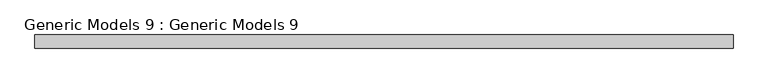
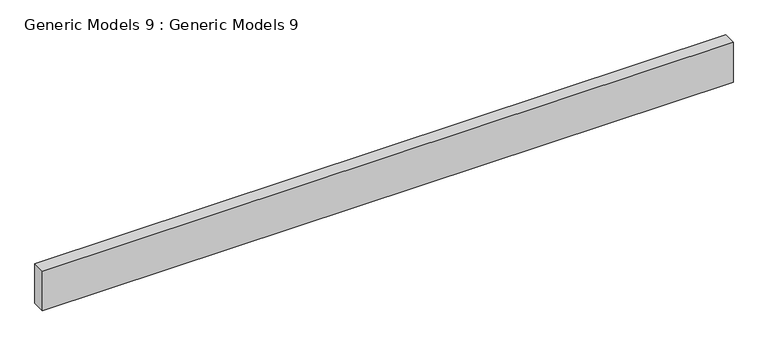
"""IFC4 building model written with IfcOpenShell, lengths in millimetres: proxy geometry, Generic Models 9 : Generic Models 9."""

from ifc_helpers import new_model, si_unit, frame, origin, place, context, project, spatial, polyline, outline, extrude, source, transform, mapped, element, save


def generic_models_9_generic_models_9_ac56366f(model_context):
    return source(origin(), model_context, "Body", "SweptSolid", [
        extrude(outline(polyline([(-19984.2998936, -1224.1526331), (-7844.1503587, -1224.1526331), (-7844.1503587, -1452.7526331), (-19984.2998936, -1452.7526331), (-19984.2998936, -1224.1526331)])), frame((0.0, 0.0, 6400.8), z_axis=(0.0, 0.0, 1.0), x_axis=(1.0, 0.0, 0.0)), (0.0, 0.0, 1.0), 737.5181991),
    ])


if __name__ == "__main__":
    model = new_model("IFC4")
    model_context = context("Model", 3, world=origin())
    ifc_project = project(units=[si_unit("LENGTHUNIT", "METRE", prefix="MILLI")], contexts=[model_context])
    site = spatial("IfcSite", under=ifc_project)
    building = spatial("IfcBuilding", under=site)
    placement = place(None, origin())
    generic_models_9_generic_models_9_shape = generic_models_9_generic_models_9_ac56366f(model_context)
    element("IfcBuildingElementProxy", 1, Name="Generic Models 9 : Generic Models 9", ObjectType="Generic Models 9 : Generic Models 9", at=placement, inside=building, context=model_context, shape_type="MappedRepresentation", body=[
        mapped(generic_models_9_generic_models_9_shape, transform((0.0, 0.0, 0.0), x_axis=(1.0, 0.0, 0.0), y_axis=(0.0, 1.0, 0.0), z_axis=(0.0, 0.0, 1.0))),
    ])
    save(model, "model.ifc")
